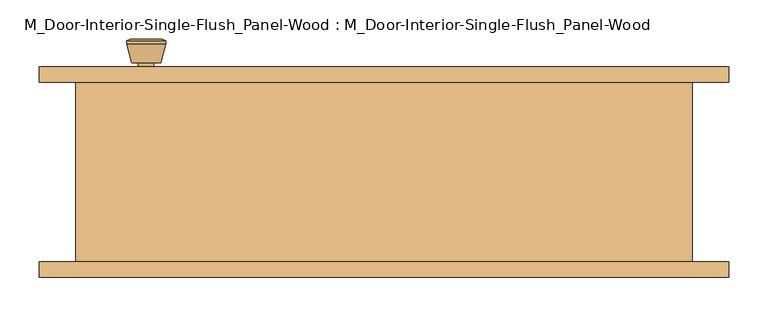
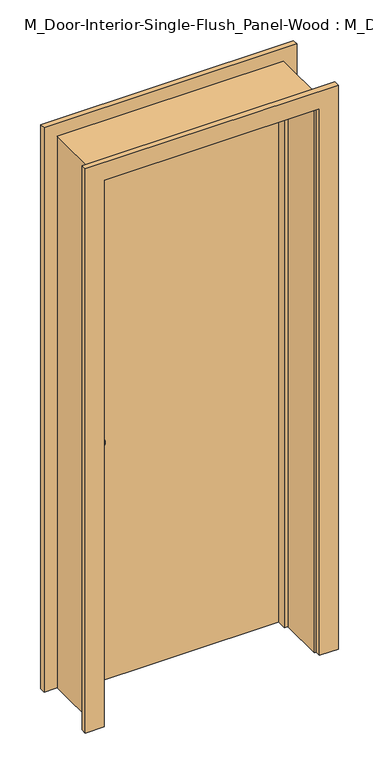
"""IFC4 building model written with IfcOpenShell, lengths in millimetres: door geometry, M_Door-Interior-Single-Flush_Panel-Wood : M_Door-Interior-Single-Flush_Panel-Wood."""

from ifc_helpers import new_model, si_unit, point, frame, frame_2d, origin, origin_with_axes, place, context, project, spatial, polyline, circle_curve, trimmed, segment, composite_curve, outline, extrude, faceted_brep, source, transform, mapped, element, save
from ifc_brep_helpers import plane_surface, cylinder_surface, revolved_surface, advanced_brep


def m_door_interior_single_flush_panel_wood_m_door_interior_542f8053(model_context):
    return source(origin(), model_context, "Body", "SolidModel", [
        advanced_brep(
        [(-303.3, 70.125, 914.4), (-293.3, 70.125, 914.4), (-313.3, 70.125, 914.4), (-282.8241324, 21.125, 914.4), (-303.3, 21.125, 914.4), (-323.7758676, 21.125, 914.4), (-278.3, 22.9528681, 914.4), (-328.3, 22.9528681, 914.4), (-278.3, 26.4165463, 914.4), (-328.3, 26.4165463, 914.4), (-284.663764, 51.125, 914.4), (-321.936236, 51.125, 914.4), (-293.3, 51.125, 914.4), (-313.3, 51.125, 914.4)],
        [
            (0, 1),
            (1, 2, circle_curve(frame((-303.3, 70.125, 914.4), z_axis=(0.0, 1.0, 0.0), x_axis=(-1.0, 0.0, 0.0)), 10.0)),
            (2, 0),
            (2, 1, circle_curve(frame((-303.3, 70.125, 914.4), z_axis=(0.0, 1.0, 0.0), x_axis=(-1.0, 0.0, 0.0)), 10.0)),
            (3, 4),
            (4, 5),
            (5, 3, circle_curve(frame((-303.3, 21.125, 914.4), z_axis=(0.0, -1.0, 0.0), x_axis=(-1.0, 0.0, 0.0)), 20.4758676)),
            (3, 5, circle_curve(frame((-303.3, 21.125, 914.4), z_axis=(0.0, -1.0, 0.0), x_axis=(-1.0, 0.0, 0.0)), 20.4758676)),
            (6, 3),
            (5, 7),
            (7, 6, circle_curve(frame((-303.3, 22.9528681, 914.4), z_axis=(0.0, -1.0, 0.0), x_axis=(-1.0, 0.0, 0.0)), 25.0)),
            (6, 7, circle_curve(frame((-303.3, 22.9528681, 914.4), z_axis=(0.0, -1.0, 0.0), x_axis=(-1.0, 0.0, 0.0)), 25.0)),
            (8, 6),
            (7, 9),
            (9, 8, circle_curve(frame((-303.3, 26.4165463, 914.4), z_axis=(0.0, -1.0, 0.0), x_axis=(-1.0, 0.0, 0.0)), 25.0)),
            (8, 9, circle_curve(frame((-303.3, 26.4165463, 914.4), z_axis=(0.0, -1.0, 0.0), x_axis=(-1.0, 0.0, 0.0)), 25.0)),
            (10, 8),
            (9, 11),
            (11, 10, circle_curve(frame((-303.3, 51.125, 914.4), z_axis=(0.0, -1.0, 0.0), x_axis=(-1.0, 0.0, 0.0)), 18.636236)),
            (10, 11, circle_curve(frame((-303.3, 51.125, 914.4), z_axis=(0.0, -1.0, 0.0), x_axis=(-1.0, 0.0, 0.0)), 18.636236)),
            (12, 10),
            (11, 13),
            (13, 12, circle_curve(frame((-303.3, 51.125, 914.4), z_axis=(0.0, -1.0, 0.0), x_axis=(-1.0, 0.0, 0.0)), 10.0)),
            (12, 13, circle_curve(frame((-303.3, 51.125, 914.4), z_axis=(0.0, -1.0, 0.0), x_axis=(-1.0, 0.0, 0.0)), 10.0)),
            (1, 12),
            (13, 2),
        ],
        [
            plane_surface(frame((-303.3, 70.125, 914.4), z_axis=(0.0, 1.0, 0.0), x_axis=(-1.0, 0.0, 0.0))),
            plane_surface(frame((-303.3, 21.125, 914.4), z_axis=(0.0, -1.0, 0.0), x_axis=(-1.0, 0.0, 0.0))),
            revolved_surface(polyline([(-323.7758676, 21.125, 914.4), (-328.3, 22.9528681, 914.4)]), (-303.3, 70.125, 914.4), (0.0, 1.0, 0.0)),
            cylinder_surface(frame((-303.3, 70.125, 914.4), z_axis=(0.0, 1.0, 0.0), x_axis=(-1.0, 0.0, 0.0)), 25.0),
            revolved_surface(polyline([(-328.3, 26.4165463, 914.4), (-321.936236, 51.125, 914.4)]), (-303.3, 70.125, 914.4), (0.0, 1.0, 0.0)),
            plane_surface(frame((-303.3, 51.125, 914.4), z_axis=(0.0, 1.0, 0.0), x_axis=(-1.0, 0.0, 0.0))),
            cylinder_surface(frame((-303.3, 70.125, 914.4), z_axis=(0.0, 1.0, 0.0), x_axis=(-1.0, 0.0, 0.0)), 10.0),
        ],
        [
            (0, [[1, 2, 3]]),
            (0, [[-3, 4, -1]]),
            (1, [[5, 6, 7]]),
            (1, [[-6, -5, 8]]),
            (2, [[9, -7, 10, 11]]),
            (2, [[-10, -8, -9, 12]]),
            (3, [[13, -11, 14, 15]]),
            (3, [[-14, -12, -13, 16]]),
            (4, [[17, -15, 18, 19]]),
            (4, [[-18, -16, -17, 20]]),
            (5, [[21, -19, 22, 23]]),
            (5, [[-22, -20, -21, 24]]),
            (6, [[25, -23, 26, -2]]),
            (6, [[-26, -24, -25, -4]]),
        ],
    ),
        extrude(outline(composite_curve([segment(trimmed(circle_curve(frame_2d((914.4, -303.3)), 30.0), [point((914.4, -333.3))], [point((914.4, -273.3))], False, "CARTESIAN"), True, "CONTINUOUS"), segment(trimmed(circle_curve(frame_2d((914.4, -303.3)), 30.0), [point((914.4, -273.3))], [point((914.4, -333.3))], False, "CARTESIAN"), True, "CONTINUOUS")], self_intersect=False)), frame((0.0, 70.125, 0.0), z_axis=(0.0, 1.0, 0.0), x_axis=(0.0, 0.0, 1.0)), (0.0, 0.0, 1.0), 6.0),
        advanced_brep(
        [(-303.3, 117.125, 914.4), (-313.3, 117.125, 914.4), (-293.3, 117.125, 914.4), (-282.8241324, 166.125, 914.4), (-323.7758676, 166.125, 914.4), (-303.3, 166.125, 914.4), (-278.3, 164.2971319, 914.4), (-328.3, 164.2971319, 914.4), (-278.3, 160.8334537, 914.4), (-328.3, 160.8334537, 914.4), (-284.663764, 136.125, 914.4), (-321.936236, 136.125, 914.4), (-293.3, 136.125, 914.4), (-313.3, 136.125, 914.4)],
        [
            (0, 1),
            (1, 2, circle_curve(frame((-303.3, 117.125, 914.4), z_axis=(0.0, -1.0, 0.0), x_axis=(-1.0, 0.0, 0.0)), 10.0)),
            (2, 0),
            (2, 1, circle_curve(frame((-303.3, 117.125, 914.4), z_axis=(0.0, -1.0, 0.0), x_axis=(-1.0, 0.0, 0.0)), 10.0)),
            (3, 4, circle_curve(frame((-303.3, 166.125, 914.4), z_axis=(0.0, 1.0, 0.0), x_axis=(-1.0, 0.0, 0.0)), 20.4758676)),
            (4, 5),
            (5, 3),
            (4, 3, circle_curve(frame((-303.3, 166.125, 914.4), z_axis=(0.0, 1.0, 0.0), x_axis=(-1.0, 0.0, 0.0)), 20.4758676)),
            (6, 7, circle_curve(frame((-303.3, 164.2971319, 914.4), z_axis=(0.0, 1.0, 0.0), x_axis=(-1.0, 0.0, 0.0)), 25.0)),
            (7, 4),
            (3, 6),
            (7, 6, circle_curve(frame((-303.3, 164.2971319, 914.4), z_axis=(0.0, 1.0, 0.0), x_axis=(-1.0, 0.0, 0.0)), 25.0)),
            (8, 9, circle_curve(frame((-303.3, 160.8334537, 914.4), z_axis=(0.0, 1.0, 0.0), x_axis=(-1.0, 0.0, 0.0)), 25.0)),
            (9, 7),
            (6, 8),
            (9, 8, circle_curve(frame((-303.3, 160.8334537, 914.4), z_axis=(0.0, 1.0, 0.0), x_axis=(-1.0, 0.0, 0.0)), 25.0)),
            (10, 11, circle_curve(frame((-303.3, 136.125, 914.4), z_axis=(0.0, 1.0, 0.0), x_axis=(-1.0, 0.0, 0.0)), 18.636236)),
            (11, 9),
            (8, 10),
            (11, 10, circle_curve(frame((-303.3, 136.125, 914.4), z_axis=(0.0, 1.0, 0.0), x_axis=(-1.0, 0.0, 0.0)), 18.636236)),
            (12, 13, circle_curve(frame((-303.3, 136.125, 914.4), z_axis=(0.0, 1.0, 0.0), x_axis=(-1.0, 0.0, 0.0)), 10.0)),
            (13, 11),
            (10, 12),
            (13, 12, circle_curve(frame((-303.3, 136.125, 914.4), z_axis=(0.0, 1.0, 0.0), x_axis=(-1.0, 0.0, 0.0)), 10.0)),
            (1, 13),
            (12, 2),
        ],
        [
            plane_surface(frame((-303.3, 117.125, 914.4), z_axis=(0.0, -1.0, 0.0), x_axis=(-1.0, 0.0, 0.0))),
            plane_surface(frame((-303.3, 166.125, 914.4), z_axis=(0.0, 1.0, 0.0), x_axis=(-1.0, 0.0, 0.0))),
            revolved_surface(polyline([(-323.7758676, 166.125, 914.4), (-328.3, 164.2971319, 914.4)]), (-303.3, 117.125, 914.4), (0.0, -1.0, 0.0)),
            cylinder_surface(frame((-303.3, 117.125, 914.4), z_axis=(0.0, -1.0, 0.0), x_axis=(-1.0, 0.0, 0.0)), 25.0),
            revolved_surface(polyline([(-328.3, 160.8334537, 914.4), (-321.936236, 136.125, 914.4)]), (-303.3, 117.125, 914.4), (0.0, -1.0, 0.0)),
            plane_surface(frame((-303.3, 136.125, 914.4), z_axis=(0.0, -1.0, 0.0), x_axis=(-1.0, 0.0, 0.0))),
            cylinder_surface(frame((-303.3, 117.125, 914.4), z_axis=(0.0, -1.0, 0.0), x_axis=(-1.0, 0.0, 0.0)), 10.0),
        ],
        [
            (0, [[1, 2, 3]]),
            (0, [[-3, 4, -1]]),
            (1, [[5, 6, 7]]),
            (1, [[8, -7, -6]]),
            (2, [[9, 10, -5, 11]]),
            (2, [[12, -11, -8, -10]]),
            (3, [[13, 14, -9, 15]]),
            (3, [[16, -15, -12, -14]]),
            (4, [[17, 18, -13, 19]]),
            (4, [[20, -19, -16, -18]]),
            (5, [[21, 22, -17, 23]]),
            (5, [[24, -23, -20, -22]]),
            (6, [[-2, 25, -21, 26]]),
            (6, [[-4, -26, -24, -25]]),
        ],
    ),
        extrude(outline(composite_curve([segment(trimmed(circle_curve(frame_2d((914.4, -303.3)), 30.0), [point((914.4, -333.3))], [point((914.4, -273.3))], False, "CARTESIAN"), True, "CONTINUOUS"), segment(trimmed(circle_curve(frame_2d((914.4, -303.3)), 30.0), [point((914.4, -273.3))], [point((914.4, -333.3))], False, "CARTESIAN"), True, "CONTINUOUS")], self_intersect=False)), frame((0.0, 111.125, 0.0), z_axis=(0.0, 1.0, 0.0), x_axis=(0.0, 0.0, 1.0)), (0.0, 0.0, 1.0), 6.0),
        faceted_brep([(393.3, 111.125, 0.0), (393.3, -117.475, 0.0), (368.3, -117.475, 0.0), (368.3, 41.2, 0.0), (355.6, 41.2, 0.0), (355.6, 76.125, 0.0), (368.3, 76.125, 0.0), (368.3, 111.125, 0.0), (393.3, 111.125, 2025.0), (393.3, -117.475, 2025.0), (-393.3, -117.475, 2025.0), (-393.3, -117.475, 0.0), (-368.3, -117.475, 0.0), (-368.3, -117.475, 2000.0), (368.3, -117.475, 2000.0), (368.3, 41.2, 2000.0), (-368.3, 41.2, 2000.0), (-368.3, 41.2, 0.0), (-355.6, 41.2, 0.0), (-355.6, 41.2, 1987.3), (355.6, 41.2, 1987.3), (355.6, 76.125, 1987.3), (-355.6, 76.125, 1987.3), (-355.6, 76.125, 0.0), (-368.3, 76.125, 0.0), (-368.3, 76.125, 2000.0), (368.3, 76.125, 2000.0), (368.3, 111.125, 2000.0), (-368.3, 111.125, 2000.0), (-368.3, 111.125, 0.0), (-393.3, 111.125, 0.0), (-393.3, 111.125, 2025.0)], [[[0, 1, 2, 3, 4, 5, 6, 7]], [[1, 0, 8, 9]], [[2, 1, 9, 10, 11, 12, 13, 14]], [[3, 2, 14, 15]], [[4, 3, 15, 16, 17, 18, 19, 20]], [[5, 4, 20, 21]], [[6, 5, 21, 22, 23, 24, 25, 26]], [[7, 6, 26, 27]], [[0, 7, 27, 28, 29, 30, 31, 8]], [[9, 8, 31, 10]], [[15, 14, 13, 16]], [[21, 20, 19, 22]], [[27, 26, 25, 28]], [[30, 29, 24, 23, 18, 17, 12, 11]], [[10, 31, 30, 11]], [[16, 13, 12, 17]], [[22, 19, 18, 23]], [[28, 25, 24, 29]]]),
        extrude(outline(polyline([(368.3, 76.125), (-368.3, 76.125), (-368.3, 111.125), (368.3, 111.125), (368.3, 76.125)])), origin_with_axes(), (0.0, 0.0, 1.0), 2000.0),
        extrude(outline(polyline([(0.0, 374.65), (0.0, 439.65), (2071.35, 439.65), (2071.35, -439.65), (0.0, -439.65), (0.0, -374.65), (2006.35, -374.65), (2006.35, 374.65), (0.0, 374.65)])), frame((0.0, 111.125, 0.0), z_axis=(0.0, 1.0, 0.0), x_axis=(0.0, 0.0, 1.0)), (0.0, 0.0, 1.0), 20.0),
        extrude(outline(polyline([(0.0, 374.65), (0.0, 439.65), (2071.35, 439.65), (2071.35, -439.65), (0.0, -439.65), (0.0, -374.65), (2006.35, -374.65), (2006.35, 374.65), (0.0, 374.65)])), frame((0.0, -137.475, 0.0), z_axis=(0.0, 1.0, 0.0), x_axis=(0.0, 0.0, 1.0)), (0.0, 0.0, 1.0), 20.0),
    ])


if __name__ == "__main__":
    model = new_model("IFC4")
    model_context = context("Model", 3, world=origin())
    ifc_project = project(units=[si_unit("LENGTHUNIT", "METRE", prefix="MILLI")], contexts=[model_context])
    site = spatial("IfcSite", under=ifc_project)
    building = spatial("IfcBuilding", under=site)
    placement = place(None, origin())
    m_door_interior_single_flush_panel_wood_m_door_interior_shape = m_door_interior_single_flush_panel_wood_m_door_interior_542f8053(model_context)
    element("IfcDoor", 1, ObjectType="M_Door-Interior-Single-Flush_Panel-Wood : M_Door-Interior-Single-Flush_Panel-Wood", at=placement, inside=building, context=model_context, shape_type="MappedRepresentation", body=[
        mapped(m_door_interior_single_flush_panel_wood_m_door_interior_shape, transform((0.0, 0.0, 0.0), x_axis=(1.0, 0.0, 0.0), y_axis=(0.0, 1.0, 0.0), z_axis=(0.0, 0.0, 1.0))),
    ])
    save(model, "model.ifc")

# Revit data of these elements
# Type "M_Door-Interior-Single-Flush_Panel-Wood : M_Door-Interior-Single-Flush_Panel-Wood"
#   Type Mark = "10"
#   Assembly Code = "C1020300"
#   Analytic Construction = "Wooden"
#   Thickness = 0' - 1.37795"
#   Thermal Resistance (R) = 2.5876 (h·ft²·°F)/BTU
#   Swing Angle [instance default] = 90.00°
#   Rough Width = 2' - 6.9685"
#   Rough Height = 6' - 7.72441"
#   Height = 6' - 6.74016"
#   Width = 2' - 5"
#   Heat Transfer Coefficient (U) = 0.3865 BTU/(h·ft²·°F)
#   Trim Material = Cherry
#   Panel Material = Cherry
#   Frame Material = Cherry
#   Door Handle Material = Aluminum
#   Visual Light Transmittance = 0
#   Solar Heat Gain Coefficient = 0
#   Wall Closure = (empty or 0)
#   Function = (empty or 0)
# Element 1 (IfcDoor, "M_Door-Interior-Single-Flush_Panel-Wood : M_Door-Interior-Single-Flush_Panel-Wood")
#   Materials on its faces: "Cherry", "Aluminum"
# Materials
#   "Cherry": class "Wood", colour RGB 226 177 128, transparency 0, Description = "Prunus Serotina", Cost = 0
#   "Aluminum": class "Metal", colour RGB 247 247 247, transparency 0, Description = "Aluminum 6061", Cost = 0
